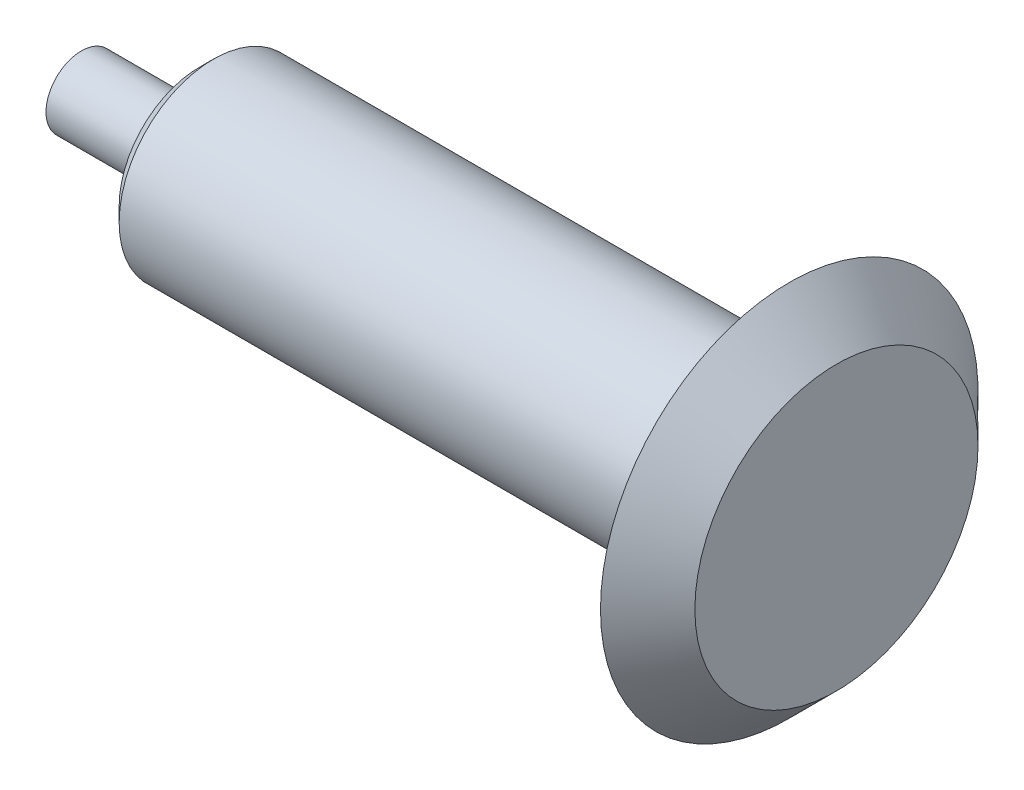
ISO-10303-21;
HEADER;
FILE_DESCRIPTION(('STEP AP214'),'2;1');
FILE_NAME('part.step','',(''),(''),'','','');
FILE_SCHEMA(('AUTOMOTIVE_DESIGN { 1 0 10303 214 1 1 1 1 }'));
ENDSEC;
DATA;
#1=APPLICATION_CONTEXT('core data for automotive mechanical design processes');
#2=APPLICATION_PROTOCOL_DEFINITION('international standard','automotive_design',2000,#1);
#3=PRODUCT_CONTEXT('',#1,'mechanical');
#4=PRODUCT('Part','Part','',(#3));
#5=PRODUCT_RELATED_PRODUCT_CATEGORY('part','',(#4));
#6=PRODUCT_DEFINITION_FORMATION('','',#4);
#7=PRODUCT_DEFINITION_CONTEXT('part definition',#1,'design');
#8=PRODUCT_DEFINITION('design','',#6,#7);
#9=PRODUCT_DEFINITION_SHAPE('','',#8);
#10=(LENGTH_UNIT() NAMED_UNIT(*) SI_UNIT(.MILLI.,.METRE.));
#11=(NAMED_UNIT(*) PLANE_ANGLE_UNIT() SI_UNIT($,.RADIAN.));
#12=(NAMED_UNIT(*) SI_UNIT($,.STERADIAN.) SOLID_ANGLE_UNIT());
#13=UNCERTAINTY_MEASURE_WITH_UNIT(LENGTH_MEASURE(1.E-05),#10,'distance_accuracy_value','');
#14=(GEOMETRIC_REPRESENTATION_CONTEXT(3) GLOBAL_UNCERTAINTY_ASSIGNED_CONTEXT((#13)) GLOBAL_UNIT_ASSIGNED_CONTEXT((#10,
#11,#12)) REPRESENTATION_CONTEXT('',''));
#15=CARTESIAN_POINT('',(0.,0.,0.));
#16=DIRECTION('',(0.,0.,1.));
#17=DIRECTION('',(1.,0.,0.));
#18=AXIS2_PLACEMENT_3D('',#15,#16,#17);
#19=CARTESIAN_POINT('',(-35.831755970441,0.,0.));
#20=DIRECTION('',(-1.,0.,0.));
#21=DIRECTION('',(0.,0.,1.));
#22=AXIS2_PLACEMENT_3D('',#19,#20,#21);
#23=PLANE('',#22);
#24=CARTESIAN_POINT('',(-35.831755970441,0.,0.));
#25=DIRECTION('',(-1.,0.,0.));
#26=DIRECTION('',(0.,0.,1.));
#27=AXIS2_PLACEMENT_3D('',#24,#25,#26);
#28=CIRCLE('',#27,7.5);
#29=CARTESIAN_POINT('',(-35.831755970441,0.,7.5));
#30=VERTEX_POINT('',#29);
#31=EDGE_CURVE('E70',#30,#30,#28,.T.);
#32=ORIENTED_EDGE('',*,*,#31,.T.);
#33=EDGE_LOOP('',(#32));
#34=FACE_BOUND('',#33,.T.);
#35=ADVANCED_FACE('F41',(#34),#23,.T.);
#36=CARTESIAN_POINT('',(124.168244029559,0.,0.));
#37=DIRECTION('',(1.,0.,0.));
#38=DIRECTION('',(0.,0.,-1.));
#39=AXIS2_PLACEMENT_3D('',#36,#37,#38);
#40=PLANE('',#39);
#41=CARTESIAN_POINT('',(124.168244029559,0.,0.));
#42=DIRECTION('',(-1.,0.,0.));
#43=DIRECTION('',(0.,0.,1.));
#44=AXIS2_PLACEMENT_3D('',#41,#42,#43);
#45=CIRCLE('',#44,29.9999999999999);
#46=CARTESIAN_POINT('',(124.168244029559,0.,29.9999999999999));
#47=VERTEX_POINT('',#46);
#48=EDGE_CURVE('E10',#47,#47,#45,.T.);
#49=ORIENTED_EDGE('',*,*,#48,.F.);
#50=EDGE_LOOP('',(#49));
#51=FACE_BOUND('',#50,.T.);
#52=ADVANCED_FACE('F88',(#51),#40,.T.);
#53=CARTESIAN_POINT('',(114.168244029559,0.,0.));
#54=DIRECTION('',(-1.,0.,0.));
#55=DIRECTION('',(0.,0.,1.));
#56=AXIS2_PLACEMENT_3D('',#53,#54,#55);
#57=CONICAL_SURFACE('',#56,40.,0.785398163397454);
#58=ORIENTED_EDGE('',*,*,#48,.T.);
#59=EDGE_LOOP('',(#58));
#60=FACE_BOUND('',#59,.T.);
#61=CARTESIAN_POINT('',(114.168244029559,0.,0.));
#62=DIRECTION('',(-1.,0.,0.));
#63=DIRECTION('',(0.,0.,1.));
#64=AXIS2_PLACEMENT_3D('',#61,#62,#63);
#65=CIRCLE('',#64,40.);
#66=CARTESIAN_POINT('',(114.168244029559,0.,40.));
#67=VERTEX_POINT('',#66);
#68=EDGE_CURVE('E50',#67,#67,#65,.T.);
#69=ORIENTED_EDGE('',*,*,#68,.F.);
#70=EDGE_LOOP('',(#69));
#71=FACE_BOUND('',#70,.T.);
#72=ADVANCED_FACE('F89',(#60,#71),#57,.T.);
#73=CARTESIAN_POINT('',(114.168244029559,0.,0.));
#74=DIRECTION('',(1.,0.,0.));
#75=DIRECTION('',(0.,0.,-1.));
#76=AXIS2_PLACEMENT_3D('',#73,#74,#75);
#77=PLANE('',#76);
#78=CARTESIAN_POINT('',(114.168244029559,0.,0.));
#79=DIRECTION('',(-1.,0.,0.));
#80=DIRECTION('',(0.,0.,1.));
#81=AXIS2_PLACEMENT_3D('',#78,#79,#80);
#82=CIRCLE('',#81,30.);
#83=CARTESIAN_POINT('',(114.168244029559,0.,30.));
#84=VERTEX_POINT('',#83);
#85=EDGE_CURVE('E51',#84,#84,#82,.T.);
#86=ORIENTED_EDGE('',*,*,#85,.F.);
#87=EDGE_LOOP('',(#86));
#88=FACE_BOUND('',#87,.T.);
#89=ORIENTED_EDGE('',*,*,#68,.T.);
#90=EDGE_LOOP('',(#89));
#91=FACE_BOUND('',#90,.T.);
#92=ADVANCED_FACE('F92',(#88,#91),#77,.F.);
#93=CARTESIAN_POINT('',(104.168244029559,0.,0.));
#94=DIRECTION('',(1.,0.,0.));
#95=DIRECTION('',(0.,0.,-1.));
#96=AXIS2_PLACEMENT_3D('',#93,#94,#95);
#97=CONICAL_SURFACE('',#96,20.,0.785398163397452);
#98=ORIENTED_EDGE('',*,*,#85,.T.);
#99=EDGE_LOOP('',(#98));
#100=FACE_BOUND('',#99,.T.);
#101=CARTESIAN_POINT('',(104.168244029559,0.,0.));
#102=DIRECTION('',(-1.,0.,0.));
#103=DIRECTION('',(0.,0.,1.));
#104=AXIS2_PLACEMENT_3D('',#101,#102,#103);
#105=CIRCLE('',#104,20.);
#106=CARTESIAN_POINT('',(104.168244029559,0.,20.));
#107=VERTEX_POINT('',#106);
#108=EDGE_CURVE('E54',#107,#107,#105,.T.);
#109=ORIENTED_EDGE('',*,*,#108,.F.);
#110=EDGE_LOOP('',(#109));
#111=FACE_BOUND('',#110,.T.);
#112=ADVANCED_FACE('F99',(#100,#111),#97,.T.);
#113=CARTESIAN_POINT('',(-51.8095123000953,0.,0.));
#114=DIRECTION('',(-1.,0.,0.));
#115=DIRECTION('',(0.,0.,1.));
#116=AXIS2_PLACEMENT_3D('',#113,#114,#115);
#117=CYLINDRICAL_SURFACE('',#116,20.);
#118=ORIENTED_EDGE('',*,*,#108,.T.);
#119=EDGE_LOOP('',(#118));
#120=FACE_BOUND('',#119,.T.);
#121=CARTESIAN_POINT('',(-7.83175597044104,0.,0.));
#122=DIRECTION('',(-1.,0.,0.));
#123=DIRECTION('',(0.,0.,1.));
#124=AXIS2_PLACEMENT_3D('',#121,#122,#123);
#125=CIRCLE('',#124,20.);
#126=CARTESIAN_POINT('',(-7.83175597044104,0.,20.));
#127=VERTEX_POINT('',#126);
#128=EDGE_CURVE('E58',#127,#127,#125,.T.);
#129=ORIENTED_EDGE('',*,*,#128,.F.);
#130=EDGE_LOOP('',(#129));
#131=FACE_BOUND('',#130,.T.);
#132=ADVANCED_FACE('F102',(#120,#131),#117,.T.);
#133=CARTESIAN_POINT('',(-7.83175597044104,0.,0.));
#134=DIRECTION('',(1.,0.,0.));
#135=DIRECTION('',(0.,0.,-1.));
#136=AXIS2_PLACEMENT_3D('',#133,#134,#135);
#137=CONICAL_SURFACE('',#136,20.,0.785398163397453);
#138=CARTESIAN_POINT('',(-10.831755970441,0.,0.));
#139=DIRECTION('',(-1.,0.,0.));
#140=DIRECTION('',(0.,0.,1.));
#141=AXIS2_PLACEMENT_3D('',#138,#139,#140);
#142=CIRCLE('',#141,17.);
#143=CARTESIAN_POINT('',(-10.831755970441,0.,17.));
#144=VERTEX_POINT('',#143);
#145=EDGE_CURVE('E64',#144,#144,#142,.T.);
#146=ORIENTED_EDGE('',*,*,#145,.F.);
#147=EDGE_LOOP('',(#146));
#148=FACE_BOUND('',#147,.T.);
#149=ORIENTED_EDGE('',*,*,#128,.T.);
#150=EDGE_LOOP('',(#149));
#151=FACE_BOUND('',#150,.T.);
#152=ADVANCED_FACE('F84',(#148,#151),#137,.T.);
#153=CARTESIAN_POINT('',(-10.831755970441,0.,0.));
#154=DIRECTION('',(-1.,0.,0.));
#155=DIRECTION('',(0.,0.,1.));
#156=AXIS2_PLACEMENT_3D('',#153,#154,#155);
#157=PLANE('',#156);
#158=ORIENTED_EDGE('',*,*,#145,.T.);
#159=EDGE_LOOP('',(#158));
#160=FACE_BOUND('',#159,.T.);
#161=CARTESIAN_POINT('',(-10.831755970441,0.,0.));
#162=DIRECTION('',(-1.,0.,0.));
#163=DIRECTION('',(0.,0.,1.));
#164=AXIS2_PLACEMENT_3D('',#161,#162,#163);
#165=CIRCLE('',#164,7.5);
#166=CARTESIAN_POINT('',(-10.831755970441,0.,7.5));
#167=VERTEX_POINT('',#166);
#168=EDGE_CURVE('E68',#167,#167,#165,.T.);
#169=ORIENTED_EDGE('',*,*,#168,.F.);
#170=EDGE_LOOP('',(#169));
#171=FACE_BOUND('',#170,.T.);
#172=ADVANCED_FACE('F77',(#160,#171),#157,.T.);
#173=CARTESIAN_POINT('',(-51.8095123000953,0.,0.));
#174=DIRECTION('',(-1.,0.,0.));
#175=DIRECTION('',(0.,0.,1.));
#176=AXIS2_PLACEMENT_3D('',#173,#174,#175);
#177=CYLINDRICAL_SURFACE('',#176,7.5);
#178=ORIENTED_EDGE('',*,*,#168,.T.);
#179=EDGE_LOOP('',(#178));
#180=FACE_BOUND('',#179,.T.);
#181=ORIENTED_EDGE('',*,*,#31,.F.);
#182=EDGE_LOOP('',(#181));
#183=FACE_BOUND('',#182,.T.);
#184=ADVANCED_FACE('F74',(#180,#183),#177,.T.);
#185=CLOSED_SHELL('',(#35,#52,#72,#92,#112,#132,#152,#172,#184));
#186=MANIFOLD_SOLID_BREP('B2',#185);
#187=ADVANCED_BREP_SHAPE_REPRESENTATION('',(#18,#186),#14);
#188=SHAPE_DEFINITION_REPRESENTATION(#9,#187);
ENDSEC;
END-ISO-10303-21;
